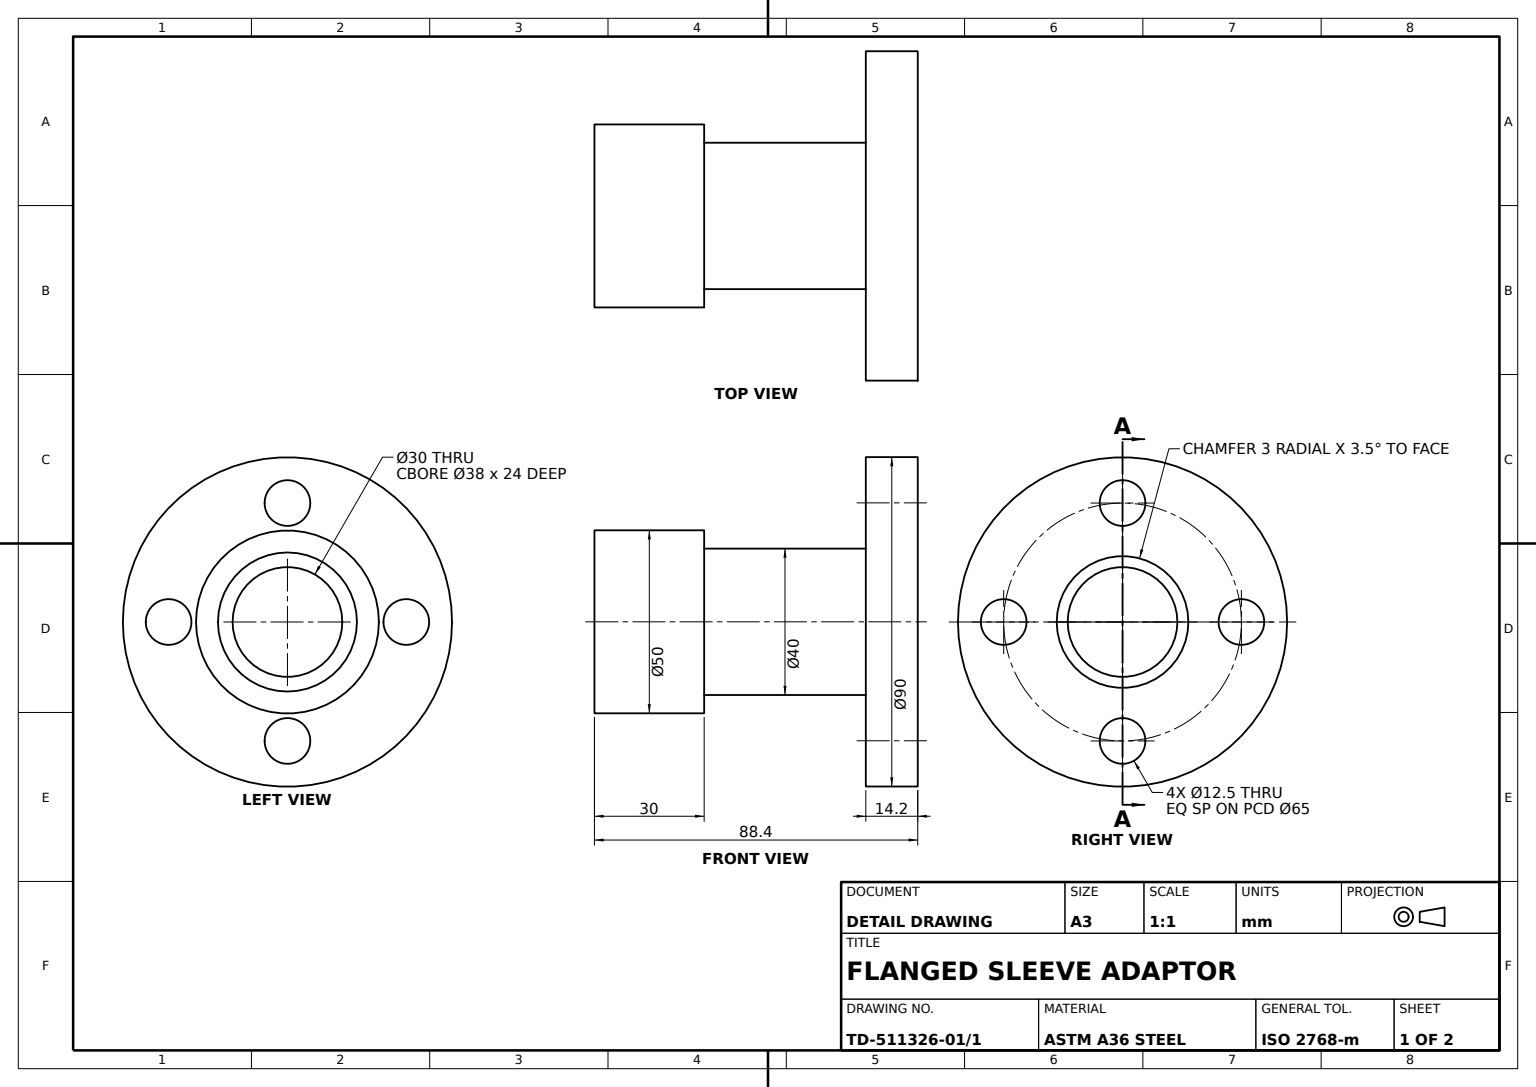
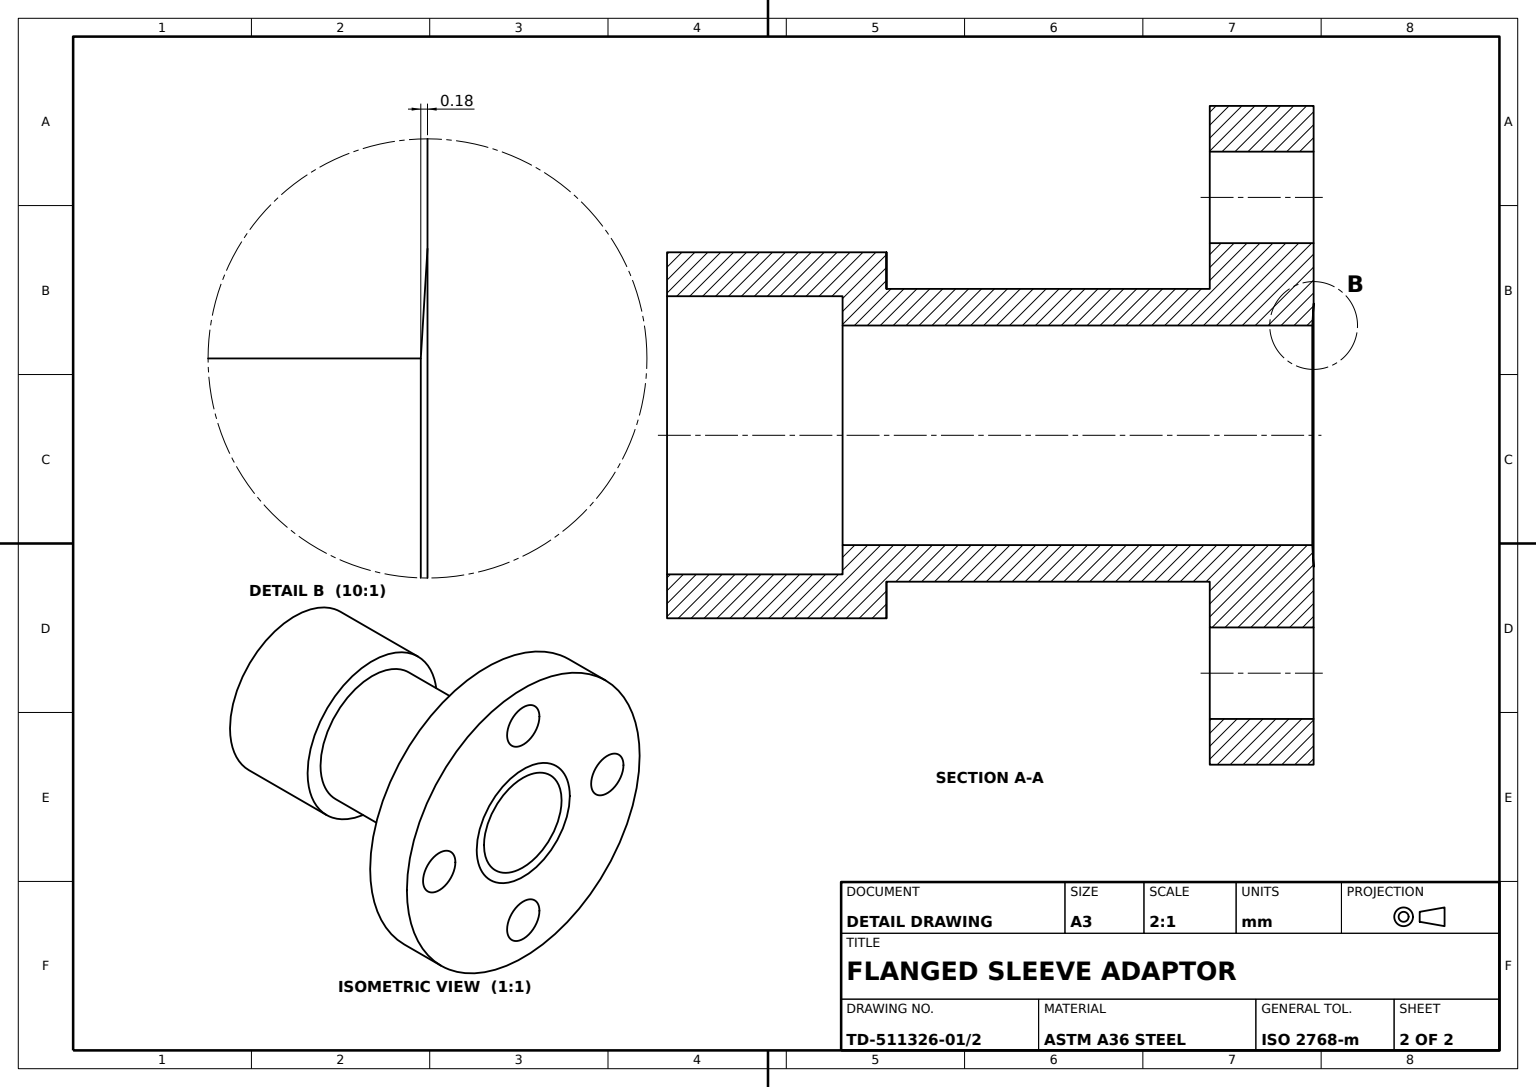
from build123d import *

# Parameters (mm, degrees)
BOLT_HOLES_SKETCH_R             = 6.25
FLANGE_BOLT_HOLES_4X_12_5_DEPTH = 98.75295392
COUNTERBORE_SKETCH_R            = 19
COUNTERBORE_38X24_DEPTH         = 24
THROUGH_BORE_30_REACH           = 110.925
THROUGH_BORE_SKETCH_R           = 15
BORE_CHAMFER_3MM_SIZE           = 3
BORE_CHAMFER_3MM_SIZE2          = 0.18348786


with BuildPart() as part:
    # Sleeve Profile Sketch → Flanged Sleeve Body (revolve)
    with BuildSketch(Plane.XY, mode=Mode.PRIVATE) as flanged_sleeve_body_sk:
        Polygon((0, 0), (0, 45), (-14.2, 45), (-14.2, 20), (-58.4, 20), (-58.4, 25), (-88.4, 25), (-88.4, 0), align=None)
    revolve(flanged_sleeve_body_sk.sketch.rotate(Axis((-88.4, 0, 0), (1, 0, 0)), 90), axis=Axis((-88.4, 0, 0), (1, 0, 0)))

    # Bolt Holes Sketch → Flange Bolt Holes 4xØ12.5 (cut, through all)
    with BuildSketch(Plane.ZY.offset(14.2)):
        with Locations((0, -32.5)):
            Circle(BOLT_HOLES_SKETCH_R)
        with Locations((-32.5, 0)):
            Circle(BOLT_HOLES_SKETCH_R)
        with Locations((0, 32.5)):
            Circle(BOLT_HOLES_SKETCH_R)
        with Locations((32.5, 0)):
            Circle(BOLT_HOLES_SKETCH_R)
    extrude(amount=-FLANGE_BOLT_HOLES_4X_12_5_DEPTH, mode=Mode.SUBTRACT)

    # Counterbore Sketch → Counterbore Ø38x24 (cut)
    with BuildSketch(Plane.ZY.offset(88.4)):
        Circle(COUNTERBORE_SKETCH_R)
    extrude(amount=-COUNTERBORE_38X24_DEPTH, mode=Mode.SUBTRACT)

    # Through Bore Sketch → Through Bore Ø30 (cut, up to next)
    with BuildSketch(Plane(origin=(0, 0, 0), x_dir=(0, 0, -1), z_dir=(1, 0, 0)), mode=Mode.PRIVATE) as through_bore_30_sk1:
        Circle(THROUGH_BORE_SKETCH_R)
    through_bore_30_tool1 = extrude(through_bore_30_sk1.sketch, amount=-THROUGH_BORE_30_REACH, mode=Mode.PRIVATE) & part.part
    add(through_bore_30_tool1.solids().sort_by_distance((0, 0, 0))[0], mode=Mode.SUBTRACT)

    # Bore Chamfer 3mm
    bore_chamfer_3mm_edges = [part.edges().sort_by_distance(p)[0] for p in [
        (0, 0, 15),
    ]]
    bore_chamfer_3mm_side = [part.faces().sort_by_distance(p)[0] for p in [
        (0, 0, -43.727207794),
    ]]
    chamfer(bore_chamfer_3mm_edges, length=BORE_CHAMFER_3MM_SIZE, length2=BORE_CHAMFER_3MM_SIZE2, reference=bore_chamfer_3mm_side[0])


solid = part.part
